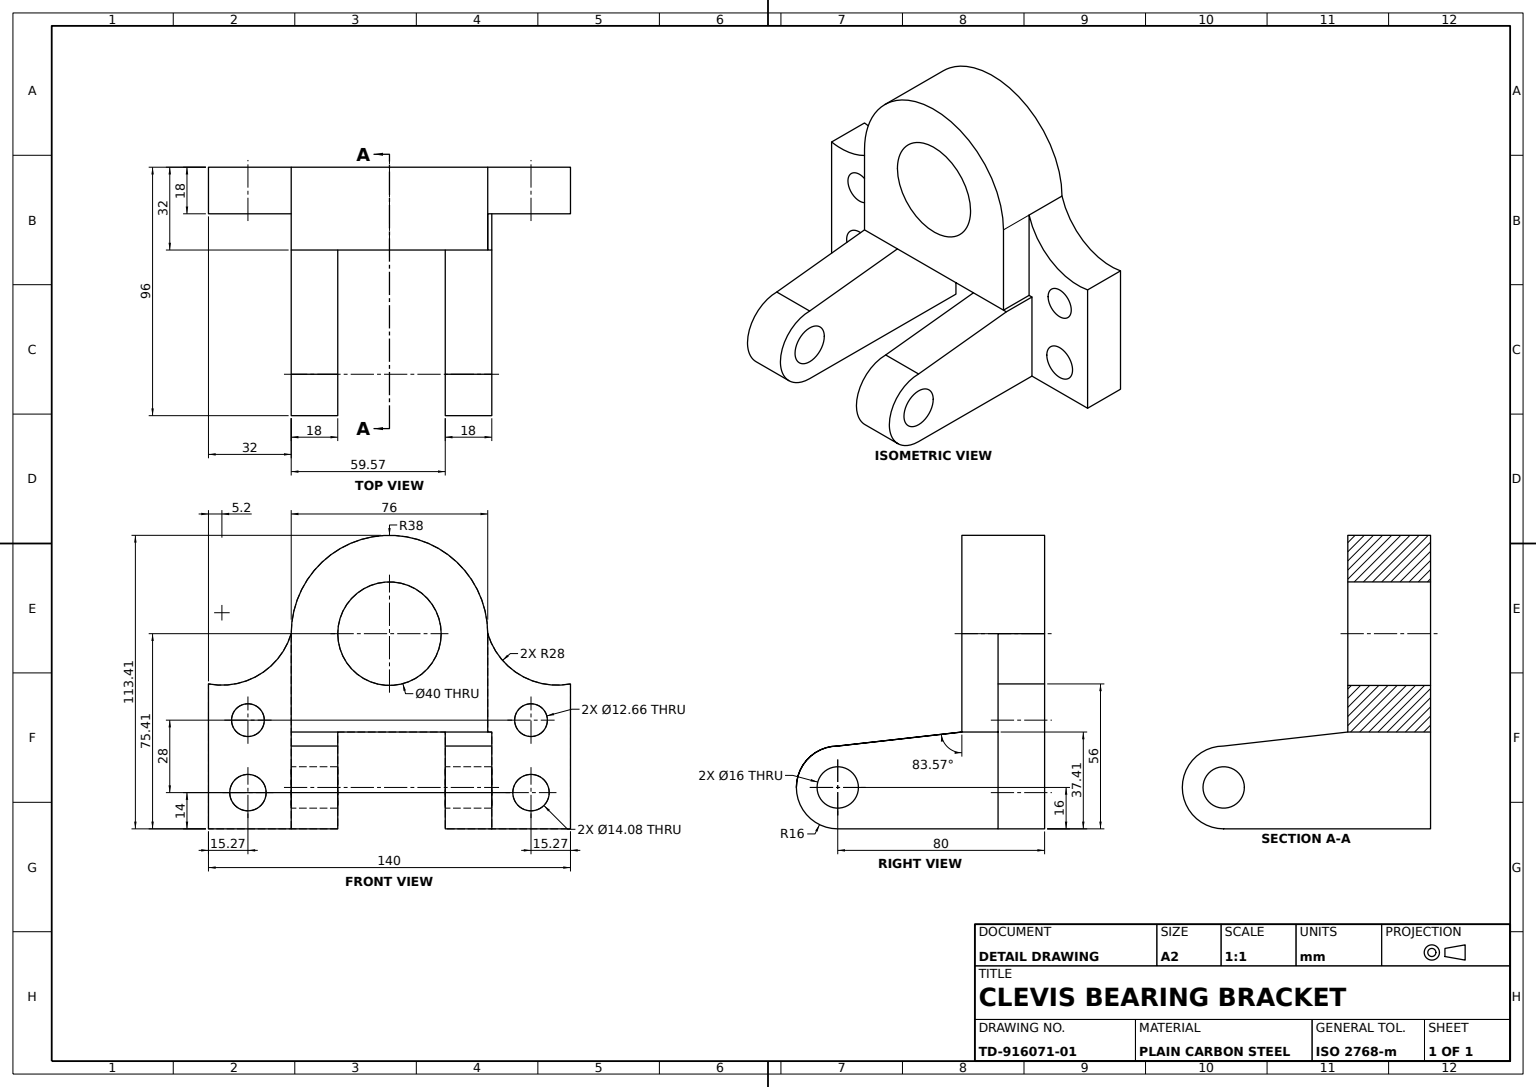
SolidWorks part; units mm, degrees
material "Plain Carbon Steel"
ref_plane "Front Plane" through (0, 0, 0) normal (0, 0, 1) x (1, 0, 0)
ref_plane "Top Plane" through (0, 0, 0) normal (0, 1, 0) x (1, 0, 0)
ref_plane "Right Plane" through (0, 0, 0) normal (1, 0, 0) x (0, 0, -1)
sketch "Hub Body Profile" plane through (0, 0, 0) normal (0, 0, 1) x (1, 0, 0)
  line L0 (134.7166, 0) -> (-149.8, 0) construction
  line L1 (0, 70.5559) -> (0, -78.8934) construction
  line L2 (0, -38) -> (38, -38)
  line L3 (0, -38) -> (-38, -38)
  line L4 (-38, -38) -> (-38, 0)
  line L5 (38, 0) -> (38, -38)
  line L6 (-38, 0) -> (-38, -74)
  line L8 (-38, -74) -> (-70, -74)
  line L11 (-70, -74) -> (-70, -18)
  line L12 (-70, 0) -> (-38, 0)
  arc A0 (38, 0) -> (-38, 0) centre (0, 0) ccw
  circle A1 centre (0, 0) radius 20
  arc A2 (-70, -18) -> (-38, 0) centre (-64.3653, 9.4272) ccw
  dimension "D1" = 76
  dimension "D2" = 40
  dimension "D6" = 28
  dimension "D3" = 74
  dimension "D4" = 32
  dimension "D5" = 56
extrude "Hub Body" add sketch "Hub Body Profile" along normal blind 32 contours L5 A0 L4 L3 L2 A1
sketch "Mounting Flange Profile" plane through (0, 0, 0) normal (0, 0, 1) x (1, 0, 0)
  line L0 (-38, 0) -> (-38, -75.4134)
  line L1 (-38, -75.4134) -> (-70, -75.4134)
  line L2 (-70, -75.4134) -> (-70, -19.4134)
  arc A0 (-70, -19.4134) -> (-38, 0) centre (-64.8028, 8.1001) ccw
  circle A1 centre (-54.7346, -33.4134) radius 6.3321
  circle A2 centre (-54.7346, -61.4134) radius 7.0401
  dimension "D1" = 28
  dimension "D4" = 14
  dimension "D6" = 12.6643
  dimension "D7" = 14.0802
  dimension "D2" = 56
  dimension "D3" = 32
  dimension "D5" = 28
  dimension "D8" = 5.1972
  dimension "D9" = 15.2654
extrude "Mounting Flange" add sketch "Mounting Flange Profile" along normal blind 18
mirror "Hub Body Mirror" about plane through (0, 0, 0) normal (1, 0, 0) of bodies 102
sketch "Clevis Arms Profile" plane through (0, 0, 0) normal (0, 0, 1) x (1, 0, 0)
  line L0 (38, -38) -> (-38, -38) construction
  line L1 (-38, -38) -> (-20, -38)
  line L2 (-38, -38) -> (-38, -75.4134)
  line L3 (-38, -75.4134) -> (-20, -75.4134)
  line L4 (-20, -38) -> (-20, -75.4134)
  line L5 (39.5716, -38) -> (21.5716, -38)
  line L6 (39.5716, -38) -> (39.5716, -75.4134)
  line L7 (39.5716, -75.4134) -> (21.5716, -75.4134)
  line L8 (21.5716, -38) -> (21.5716, -75.4134)
  dimension "D1" = 18
  dimension "D2" = 18
  dimension "D3" = 59.5716
  dimension "D4" = 37.4134
extrude "Clevis Arms" add sketch "Clevis Arms Profile" along normal blind 96
sketch "Clevis Slot Profile" plane through (-38, 0, 0) normal (-1, 0, 0) x (0, 0, 1)
  line L0 (96, -75.4134) -> (18, -75.4134) construction
  line L1 (0, -19.4134) -> (0, -75.4134) construction
  line L2 (80, -43.4134) -> (32, -38)
  circle A0 centre (80, -59.4134) radius 8
  circle A1 centre (80, -59.4134) radius 16
  dimension "D1" = 16
  dimension "D2" = 32
  dimension "D4" = 16
  dimension "D3" = 80
extrude "Clevis Slot Cut" cut sketch "Clevis Slot Profile" against normal through all contours A0 | A1 A0 L2 | A1 L2 A0
